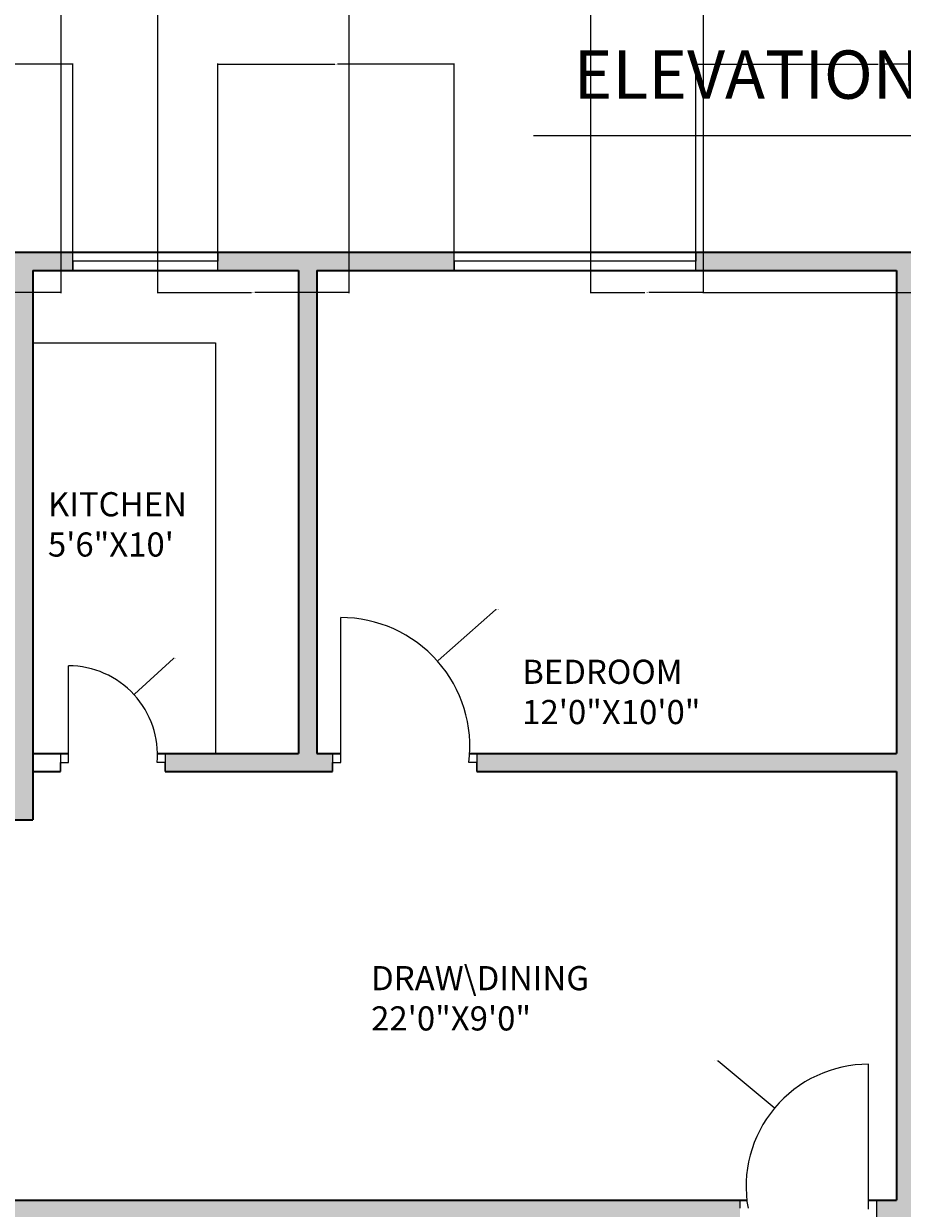
# Model space of a CAD drawing. Units: inches. Extents: x 2314 to 3223, y 1382 to 2735.
# Tile 9 of 14: x 2549 to 2767, y 2144 to 2439. Entities that reach past the tile are written whole.
import ezdxf

# ---------------------------------------------------------------- set-up
doc = ezdxf.new("R2010")
doc.units = ezdxf.units.IN
for name, color, linetype, lineweight in [('A-ANNO-DIMS', 2, 'Continuous', 18), ('A-ANNO-TEXT', 7, 'Continuous', 25), ('A-AREA-IDEN', 7, 'Continuous', 18), ('A-DOOR', 3, 'Continuous', 18), ('A-FLOR-FIXT', 8, 'Continuous', 18), ('A-GLAZ', 4, 'Continuous', 18), ('A-WALL', 7, 'Continuous', 35)]:
    doc.layers.add(name, color=color, linetype=linetype, lineweight=lineweight)
doc.layers.add('A-WALL-PATT', color=251, linetype='Continuous', lineweight=13, true_color=0x636466)
doc.styles.get("Standard").update_dxf_attribs({"font": 'arial.ttf'})
doc.dimstyles.get("Standard").update_dxf_attribs({"dimtxt": 0.18, "dimasz": 0.18, "dimexe": 0.18, "dimexo": 0.0625, "dimgap": 0.09, "dimtad": 0, "dimtih": 1, "dimtoh": 1, "dimdec": 4, "dimzin": 0, "dimdsep": 46, "dimtxsty": 'Standard', "dimcen": 0.09, "dimadec": 0, "dimazin": 0, "dimtfac": 1, "dimtdec": 4, "dimtofl": 0, "dimtmove": 0, "dimatfit": 3, "dimfxl": 1, "dimtolj": 1, "dimtzin": 0, "dimarcsym": 0})

# ---------------------------------------------------------------- blocks, each defined once
blk = doc.blocks.new('WIN-PLAN-60')
for p, q in [((0, 4.5), (0, 0)), ((60, 2.25), (60, 4.5)), ((60, 4.5), (60, 0)), ((0, 0), (0, 2.25)), ((0, 2.25), (60, 2.25))]:
    blk.add_line(p, q)
blk = doc.blocks.new('WIN-PLAN-36')
for p, q in [((0, 36), (4.5, 36)), ((4.5, 36), (2.25, 36)), ((2.25, 36), (2.25, 0)), ((2.25, 0), (0, 0)), ((0, 0), (4.5, 0))]:
    blk.add_line(p, q)
blk = doc.blocks.new('*D41')
at = {"layer": 'A-ANNO-DIMS', "color": 0, "lineweight": -2, "transparency": 16777216}
for p, q in [((2503.33, 2381.85), (2503.33, 2428.66)), ((2503.51, 2428.48), (2531.95, 2428.48)), ((2561.18, 2428.48), (2532.74, 2428.48)), ((2561.36, 2381.85), (2561.36, 2428.66))]:
    blk.add_line(p, q, dxfattribs=at)
at = {"layer": 'A-ANNO-DIMS', "color": 0, "transparency": 16777216}
for points in [[(2503.51, 2428.51), (2503.51, 2428.45), (2503.33, 2428.48)], [(2561.18, 2428.51), (2561.18, 2428.45), (2561.36, 2428.48)]]:
    blk.add_solid(points, dxfattribs=at)
at = {"layer": 'Defpoints', "color": 0, "transparency": 16777216}
for p in [(2561.36, 2428.48), (2503.33, 2381.78), (2561.36, 2381.78)]:
    blk.add_point(p, dxfattribs=at)
at = {"layer": 'A-ANNO-DIMS', "color": 0, "transparency": 16777216, "insert": (2532.35, 2428.48), "char_height": 0.18, "attachment_point": 5}
blk.add_mtext('\\A1;58.03', dxfattribs=at)
blk = doc.blocks.new('*D42')
at = {"layer": 'A-ANNO-DIMS', "color": 0, "lineweight": -2, "transparency": 16777216}
for p, q in [((2597.36, 2381.85), (2597.36, 2428.66)), ((2597.54, 2428.48), (2626.39, 2428.48)), ((2655.88, 2428.48), (2627.04, 2428.48)), ((2656.06, 2381.85), (2656.06, 2428.66))]:
    blk.add_line(p, q, dxfattribs=at)
at = {"layer": 'A-ANNO-DIMS', "color": 0, "transparency": 16777216}
for points in [[(2597.54, 2428.51), (2597.54, 2428.45), (2597.36, 2428.48)], [(2655.88, 2428.51), (2655.88, 2428.45), (2656.06, 2428.48)]]:
    blk.add_solid(points, dxfattribs=at)
at = {"layer": 'Defpoints', "color": 0, "transparency": 16777216}
for p in [(2656.06, 2428.48), (2597.36, 2381.78), (2656.06, 2381.78)]:
    blk.add_point(p, dxfattribs=at)
at = {"layer": 'A-ANNO-DIMS', "color": 0, "transparency": 16777216, "insert": (2626.71, 2428.48), "char_height": 0.18, "attachment_point": 5}
blk.add_mtext('\\A1;58.7', dxfattribs=at)
blk = doc.blocks.new('*D43')
at = {"layer": 'A-ANNO-DIMS', "color": 0, "lineweight": -2, "transparency": 16777216}
for p, q in [((2716.06, 2381.85), (2716.06, 2428.66)), ((2716.24, 2428.48), (2761.31, 2428.48)), ((2807.16, 2428.48), (2762.1, 2428.48)), ((2807.34, 2381.85), (2807.34, 2428.66))]:
    blk.add_line(p, q, dxfattribs=at)
at = {"layer": 'A-ANNO-DIMS', "color": 0, "transparency": 16777216}
for points in [[(2716.24, 2428.51), (2716.24, 2428.45), (2716.06, 2428.48)], [(2807.16, 2428.51), (2807.16, 2428.45), (2807.34, 2428.48)]]:
    blk.add_solid(points, dxfattribs=at)
at = {"layer": 'Defpoints', "color": 0, "transparency": 16777216}
for p in [(2807.34, 2428.48), (2716.06, 2381.78), (2807.34, 2381.78)]:
    blk.add_point(p, dxfattribs=at)
at = {"layer": 'A-ANNO-DIMS', "color": 0, "transparency": 16777216, "insert": (2761.7, 2428.48), "char_height": 0.18, "attachment_point": 5}
blk.add_mtext('\\A1;91.28', dxfattribs=at)
blk = doc.blocks.new('*D53')
at = {"layer": 'A-ANNO-DIMS', "color": 0, "lineweight": -2, "transparency": 16777216}
for p, q in [((2502.93, 2502.62), (2502.93, 2371.63)), ((2558.38, 2502.62), (2558.38, 2371.63)), ((2503.11, 2371.81), (2530.26, 2371.81)), ((2558.2, 2371.81), (2531.05, 2371.81))]:
    blk.add_line(p, q, dxfattribs=at)
at = {"layer": 'A-ANNO-DIMS', "color": 0, "transparency": 16777216}
for points in [[(2503.11, 2371.84), (2503.11, 2371.78), (2502.93, 2371.81)], [(2558.2, 2371.84), (2558.2, 2371.78), (2558.38, 2371.81)]]:
    blk.add_solid(points, dxfattribs=at)
at = {"layer": 'Defpoints', "color": 0, "transparency": 16777216}
for p in [(2502.93, 2502.68), (2558.38, 2502.68), (2558.38, 2371.81)]:
    blk.add_point(p, dxfattribs=at)
at = {"layer": 'A-ANNO-DIMS', "color": 0, "transparency": 16777216, "insert": (2530.66, 2371.81), "char_height": 0.18, "attachment_point": 5}
blk.add_mtext('\\A1;55.45', dxfattribs=at)
blk = doc.blocks.new('*D54')
at = {"layer": 'A-ANNO-DIMS', "color": 0, "lineweight": -2, "transparency": 16777216}
for p, q in [((2582.38, 2502.62), (2582.38, 2371.63)), ((2629.85, 2502.62), (2629.85, 2371.63)), ((2582.56, 2371.81), (2605.72, 2371.81)), ((2629.67, 2371.81), (2606.51, 2371.81))]:
    blk.add_line(p, q, dxfattribs=at)
at = {"layer": 'A-ANNO-DIMS', "color": 0, "transparency": 16777216}
for points in [[(2582.56, 2371.84), (2582.56, 2371.78), (2582.38, 2371.81)], [(2629.67, 2371.84), (2629.67, 2371.78), (2629.85, 2371.81)]]:
    blk.add_solid(points, dxfattribs=at)
at = {"layer": 'Defpoints', "color": 0, "transparency": 16777216}
for p in [(2582.38, 2502.68), (2629.85, 2502.68), (2629.85, 2371.81)]:
    blk.add_point(p, dxfattribs=at)
at = {"layer": 'A-ANNO-DIMS', "color": 0, "transparency": 16777216, "insert": (2606.11, 2371.81), "char_height": 0.18, "attachment_point": 5}
blk.add_mtext('\\A1;47.47', dxfattribs=at)
blk = doc.blocks.new('*D55')
at = {"layer": 'A-ANNO-DIMS', "color": 0, "lineweight": -2, "transparency": 16777216}
for p, q in [((2689.85, 2502.62), (2689.85, 2371.63)), ((2717.89, 2466.62), (2717.89, 2371.63)), ((2690.03, 2371.81), (2703.4, 2371.81)), ((2717.71, 2371.81), (2704.33, 2371.81))]:
    blk.add_line(p, q, dxfattribs=at)
at = {"layer": 'A-ANNO-DIMS', "color": 0, "transparency": 16777216}
for points in [[(2690.03, 2371.84), (2690.03, 2371.78), (2689.85, 2371.81)], [(2717.71, 2371.84), (2717.71, 2371.78), (2717.89, 2371.81)]]:
    blk.add_solid(points, dxfattribs=at)
at = {"layer": 'Defpoints', "color": 0, "transparency": 16777216}
for p in [(2689.85, 2502.68), (2717.89, 2466.68), (2717.89, 2371.81)]:
    blk.add_point(p, dxfattribs=at)
at = {"layer": 'A-ANNO-DIMS', "color": 0, "transparency": 16777216, "insert": (2703.87, 2371.81), "char_height": 0.18, "attachment_point": 5}
blk.add_mtext('\\A1;28.046', dxfattribs=at)
blk = doc.blocks.new('*D56')
at = {"layer": 'A-ANNO-DIMS', "color": 0, "lineweight": -2, "transparency": 16777216}
for p, q in [((2717.89, 2466.62), (2717.89, 2371.63)), ((2822.89, 2466.62), (2822.89, 2371.63)), ((2718.07, 2371.81), (2770.11, 2371.81)), ((2822.71, 2371.81), (2770.67, 2371.81))]:
    blk.add_line(p, q, dxfattribs=at)
at = {"layer": 'A-ANNO-DIMS', "color": 0, "transparency": 16777216}
for points in [[(2718.07, 2371.84), (2718.07, 2371.78), (2717.89, 2371.81)], [(2822.71, 2371.84), (2822.71, 2371.78), (2822.89, 2371.81)]]:
    blk.add_solid(points, dxfattribs=at)
at = {"layer": 'Defpoints', "color": 0, "transparency": 16777216}
for p in [(2717.89, 2466.68), (2822.89, 2466.68), (2822.89, 2371.81)]:
    blk.add_point(p, dxfattribs=at)
at = {"layer": 'A-ANNO-DIMS', "color": 0, "transparency": 16777216, "insert": (2770.39, 2371.81), "char_height": 0.18, "attachment_point": 5}
blk.add_mtext('\\A1;105', dxfattribs=at)
blk = doc.blocks.new('*D66')
at = {"layer": 'A-ANNO-DIMS', "color": 0, "lineweight": -2, "transparency": 16777216}
for p, q in [((2666.3, 2292.96), (2652.02, 2280.33)), ((2666.48, 2292.96), (2666.3, 2292.96)), ((2627.76, 2258.95), (2627.94, 2258.95)), ((2627.85, 2258.86), (2627.85, 2259.04))]:
    blk.add_line(p, q, dxfattribs=at)
at = {"layer": 'A-ANNO-DIMS', "color": 0, "transparency": 16777216}
blk.add_solid([(2652, 2280.35), (2652.04, 2280.3), (2651.88, 2280.21)], dxfattribs=at)
at = {"layer": 'Defpoints', "color": 0, "transparency": 16777216}
for p in [(2651.88, 2280.21), (2627.85, 2258.95)]:
    blk.add_point(p, dxfattribs=at)
at = {"layer": 'A-ANNO-DIMS', "color": 0, "transparency": 16777216, "insert": (2666.96, 2292.96), "char_height": 0.18, "attachment_point": 5}
blk.add_mtext('\\A1;R32.08', dxfattribs=at)
blk = doc.blocks.new('*D68')
at = {"layer": 'A-ANNO-DIMS', "color": 0, "lineweight": -2, "transparency": 16777216}
for p, q in [((2721.4, 2180.88), (2721.58, 2180.88)), ((2721.58, 2180.88), (2735.45, 2169.29)), ((2758.84, 2149.66), (2759.02, 2149.66)), ((2758.93, 2149.57), (2758.93, 2149.75))]:
    blk.add_line(p, q, dxfattribs=at)
at = {"layer": 'A-ANNO-DIMS', "color": 0, "transparency": 16777216}
blk.add_solid([(2735.47, 2169.31), (2735.43, 2169.27), (2735.59, 2169.17)], dxfattribs=at)
at = {"layer": 'Defpoints', "color": 0, "transparency": 16777216}
for p in [(2735.59, 2169.17), (2758.93, 2149.66)]:
    blk.add_point(p, dxfattribs=at)
at = {"layer": 'A-ANNO-DIMS', "color": 0, "transparency": 16777216, "insert": (2720.92, 2180.88), "char_height": 0.18, "attachment_point": 5}
blk.add_mtext('\\A1;R30.42', dxfattribs=at)
blk = doc.blocks.new('*D85')
at = {"layer": 'A-ANNO-DIMS', "color": 0, "lineweight": -2, "transparency": 16777216}
for p, q in [((2586.3, 2280.82), (2576.67, 2271.99)), ((2586.48, 2280.82), (2586.3, 2280.82)), ((2560.17, 2256.96), (2560.35, 2256.96)), ((2560.26, 2256.87), (2560.26, 2257.05))]:
    blk.add_line(p, q, dxfattribs=at)
at = {"layer": 'A-ANNO-DIMS', "color": 0, "transparency": 16777216}
blk.add_solid([(2576.65, 2272.02), (2576.69, 2271.97), (2576.54, 2271.87)], dxfattribs=at)
at = {"layer": 'Defpoints', "color": 0, "transparency": 16777216}
for p in [(2576.54, 2271.87), (2560.26, 2256.96)]:
    blk.add_point(p, dxfattribs=at)
at = {"layer": 'A-ANNO-DIMS', "color": 0, "transparency": 16777216, "insert": (2587.03, 2280.82), "char_height": 0.18, "attachment_point": 5}
blk.add_mtext('\\A1;R22.075', dxfattribs=at)

msp = doc.modelspace()

# ---------------------------------------------------------------- hatches: boundary and pattern name
at = {"layer": 'A-WALL-PATT'}
h = msp.add_hatch(color=256, dxfattribs=at)
h.dxf.hatch_style = 1
h.paths.add_polyline_path([(2443.3302, 2379.5332), (2443.3302, 2381.7832), (2410.3927, 2381.7832), (2410.3927, 2336.7008), (2414.8927, 2336.7008), (2414.8927, 2377.2832), (2443.3302, 2377.2832)])
h.paths.add_polyline_path([(2561.3645, 2379.5332), (2561.3645, 2381.7832), (2503.3302, 2381.7832), (2503.3302, 2377.2832), (2546.8927, 2377.2832), (2546.8927, 2245.2832), (2541.8787, 2245.2832), (2541.8787, 2240.7832), (2551.3927, 2240.7832), (2551.3927, 2377.2832), (2561.3645, 2377.2832)])
h.paths.add_polyline_path([(2656.0607, 2381.7832), (2597.3645, 2381.7832), (2597.3645, 2377.2832), (2617.3927, 2377.2832), (2617.3927, 2257.2832), (2584.2532, 2257.2832), (2584.2532, 2252.7832), (2625.8528, 2252.7832), (2625.8528, 2255.0332), (2625.8528, 2257.2832), (2621.8927, 2257.2832), (2621.8927, 2377.2832), (2656.0607, 2377.2832), (2656.0607, 2379.5332)])
h.paths.add_polyline_path([(2807.3418, 2381.7832), (2716.0607, 2381.7832), (2716.0607, 2377.2832), (2765.8927, 2377.2832), (2765.8927, 2257.2832), (2661.6935, 2257.2832), (2661.6935, 2252.7832), (2765.8927, 2252.7832), (2765.8927, 2146.2832), (2760.9259, 2146.2832), (2760.9259, 2141.8832), (2775.7119, 2141.8832), (2775.7119, 2146.2832), (2770.3927, 2146.2832), (2770.3927, 2252.7832), (2877.684, 2252.7832), (2877.684, 2255.0332), (2877.684, 2257.2832), (2770.3927, 2257.2832), (2770.3927, 2377.2832), (2807.3418, 2377.2832), (2807.3418, 2379.5332)])
h.paths.add_polyline_path([(2937.2118, 2381.7832), (2867.3418, 2381.7832), (2867.3418, 2377.2832), (2914.3927, 2377.2832), (2914.3927, 2257.2832), (2908.4124, 2257.2832), (2908.4124, 2252.7832), (2960.6432, 2252.7832), (2960.6432, 2255.0332), (2960.6432, 2257.2832), (2918.8927, 2257.2832), (2918.8927, 2377.2832), (2937.2118, 2377.2832)])
h.paths.add_polyline_path([(3022.1601, 2381.7832), (2973.2118, 2381.7832), (2973.2118, 2379.5332), (2973.2118, 2377.2832), (2984.8927, 2377.2832), (2984.8927, 2257.2832), (2980.0601, 2257.2832), (2980.0601, 2252.7832), (2984.8927, 2252.7832), (2984.8927, 2240.7832), (2995.668, 2240.7832), (2995.668, 2243.0332), (2995.668, 2245.2832), (2989.3927, 2245.2832), (2989.3927, 2377.2832), (3022.1601, 2377.2832), (3022.1601, 2379.5332)])
h.paths.add_polyline_path([(3125.8927, 2381.7832), (3082.1601, 2381.7832), (3082.1601, 2377.2832), (3121.3927, 2377.2832), (3121.3927, 2334.7388), (3125.8927, 2334.7388)])
h.paths.add_polyline_path([(3125.8927, 2274.7388), (3121.3927, 2274.7388), (3121.3927, 2245.2832), (3066.4832, 2245.2832), (3066.4832, 2240.7832), (3121.3927, 2240.7832), (3121.3927, 2232.1868), (3125.8927, 2232.1868)])
h.paths.add_polyline_path([(3125.8927, 2208.1868), (3121.3927, 2208.1868), (3121.3927, 2198.7832), (3037.3927, 2198.7832), (3037.3927, 2240.7832), (3041.2694, 2240.7832), (3041.2694, 2243.0332), (3041.2694, 2245.2832), (3026.8205, 2245.2832), (3026.8205, 2240.7832), (3032.8927, 2240.7832), (3032.8927, 2190.4022), (3037.3927, 2190.4022), (3037.3927, 2194.2832), (3121.3927, 2194.2832), (3121.3927, 2182.1835), (3125.8927, 2182.1835)])
h.paths.add_polyline_path([(3125.8927, 2158.1835), (3121.3927, 2158.1835), (3121.3927, 2146.2832), (3037.3927, 2146.2832), (3037.3927, 2169.3726), (3035.1427, 2169.3726), (3032.8927, 2169.3726), (3032.8927, 2146.2832), (2812.7301, 2146.2832), (2812.7301, 2144.0832), (2812.7301, 2141.8832), (2818.3927, 2141.8832), (2818.3927, 1970.1316), (2822.8927, 1970.1316), (2822.8927, 1978.8832), (2903.9846, 1978.8832), (2903.9846, 1981.1332), (2903.9846, 1983.3832), (2822.8927, 1983.3832), (2822.8927, 2115.3832), (2851.7162, 2115.3832), (2851.7162, 2117.6332), (2851.7162, 2119.8832), (2822.8927, 2119.8832), (2822.8927, 2141.8832), (3125.8927, 2141.8832)])
h.paths.add_polyline_path([(3125.8927, 2119.8832), (3081.193, 2119.8832), (3081.193, 2115.3832), (3121.3927, 2115.3832), (3121.3927, 2071.8188), (3125.8927, 2071.8188)], flags=17)
h.paths.add_polyline_path([(2989.3927, 2115.3832), (3021.193, 2115.3832), (3021.193, 2117.6332), (3021.193, 2119.8832), (2979.123, 2119.8832), (2979.123, 2115.3832), (2984.8927, 2115.3832), (2984.8927, 2019.3832), (2981.9225, 2019.3832), (2981.9225, 2014.8832), (2984.8927, 2014.8832), (2984.8927, 1983.3832), (2984.8927, 1978.8832), (2989.3927, 1978.8832), (2989.3927, 1983.3832)], flags=17)
h.paths.add_polyline_path([(2947.3927, 2115.3832), (2955.123, 2115.3832), (2955.123, 2117.6332), (2955.123, 2119.8832), (2911.7162, 2119.8832), (2911.7162, 2115.3832), (2942.8927, 2115.3832), (2942.8927, 1983.3832), (2936.7017, 1983.3832), (2936.7017, 1978.8832), (2947.3927, 1978.8832), (2947.3927, 1983.3832), (2947.3927, 2014.8832), (2960.7167, 2014.8832), (2960.7167, 2017.1332), (2960.7167, 2019.3832), (2947.3927, 2019.3832)], flags=17)
h.paths.add_polyline_path([(3037.3927, 1978.8832), (3041.8276, 1978.8832), (3041.8276, 1981.1332), (3041.8276, 1983.3832), (3025.477, 1983.3832), (3025.477, 1978.8832), (3032.8927, 1978.8832), (3032.8927, 1927.1259), (3035.1427, 1927.1259), (3037.3927, 1927.1259)])
h.paths.add_polyline_path([(3125.8927, 2011.8188), (3123.6427, 2011.8188), (3121.3927, 2011.8188), (3121.3927, 1983.3832), (3065, 1983.3832), (3065, 1978.8832), (3121.3927, 1978.8832), (3121.3927, 1970.5932), (3125.8927, 1970.5932)], flags=17)
h.paths.add_polyline_path([(2994.2341, 1983.3832), (2989.3927, 1983.3832), (2989.3927, 1978.8832), (2994.2341, 1978.8832), (2994.2341, 1981.1332)], flags=16)
h.paths.add_polyline_path([(3125.8927, 1946.5932), (3121.3927, 1946.5932), (3121.3927, 1936.8832), (3037.3927, 1936.8832), (3037.3927, 1932.3832), (3121.3927, 1932.3832), (3121.3927, 1919.825), (3125.8927, 1919.825)])
h.paths.add_polyline_path([(3125.8927, 1883.825), (3121.3927, 1883.825), (3121.3927, 1866.3832), (3037.3927, 1866.3832), (3037.3927, 1899.0954), (3035.1427, 1899.0954), (3032.8927, 1899.0954), (3032.8927, 1866.3832), (2822.8927, 1866.3832), (2822.8927, 1938.7212), (2820.6427, 1938.7212), (2818.3927, 1938.7212), (2818.3927, 1786.9239), (2822.8927, 1786.9239), (2822.8927, 1861.8832), (3032.8927, 1861.8832), (3032.8927, 1825.1023), (3037.3927, 1825.1023), (3037.3927, 1861.8832), (3121.3927, 1861.8832), (3121.3927, 1844.6765), (3125.8927, 1844.6765)])
h.paths.add_polyline_path([(3125.8927, 1808.6765), (3121.3927, 1808.6765), (3121.3927, 1795.8832), (3037.3927, 1795.8832), (3037.3927, 1799.4755), (3032.8927, 1799.4755), (3032.8927, 1749.3832), (3026.5034, 1749.3832), (3026.5034, 1744.8832), (3032.8927, 1744.8832), (3034.9255, 1744.8832), (3043.1326, 1744.8832), (3043.1326, 1747.1332), (3043.1326, 1749.3832), (3037.3927, 1749.3832), (3037.3927, 1791.3832), (3121.3927, 1791.3832), (3121.3927, 1783.3103), (3125.8927, 1783.3103)])
h.paths.add_polyline_path([(3125.8927, 1759.3103), (3121.3927, 1759.3103), (3121.3927, 1749.3832), (3065.1845, 1749.3832), (3065.1845, 1744.8832), (3121.3927, 1744.8832), (3121.3927, 1709.3573), (3125.8927, 1709.3573)])
h.paths.add_polyline_path([(3125.8927, 1649.3573), (3121.3927, 1649.3573), (3121.3927, 1612.8832), (3095.116, 1612.8832), (3095.116, 1608.3832), (3125.8927, 1608.3832)])
h.paths.add_polyline_path([(3035.116, 1612.8832), (2993.8927, 1612.8832), (2993.8927, 1744.8832), (2998.7409, 1744.8832), (2998.7409, 1749.3832), (2989.3927, 1749.3832), (2989.3927, 1744.8832), (2989.3927, 1701.3832), (2972.8226, 1701.3832), (2972.8226, 1696.8832), (2989.3927, 1696.8832), (2989.3927, 1612.8832), (2978.2225, 1612.8832), (2978.2225, 1608.3832), (3035.116, 1608.3832), (3035.116, 1610.6332)])
h.paths.add_polyline_path([(2947.3927, 1696.8832), (2950.7566, 1696.8832), (2950.7566, 1699.1332), (2950.7566, 1701.3832), (2947.3927, 1701.3832), (2947.3927, 1744.8832), (2947.3927, 1749.3832), (2937.649, 1749.3832), (2937.649, 1744.8832), (2942.8927, 1744.8832), (2942.8927, 1612.8832), (2907.783, 1612.8832), (2907.783, 1608.3832), (2954.2225, 1608.3832), (2954.2225, 1610.6332), (2954.2225, 1612.8832), (2947.3927, 1612.8832)])
h.paths.add_polyline_path([(2822.8927, 1744.8832), (2905.3491, 1744.8832), (2905.3491, 1747.1332), (2905.3491, 1749.3832), (2822.8927, 1749.3832), (2822.8927, 1756.9185), (2818.3927, 1756.9185), (2818.3927, 1612.8832), (2818.3927, 1569.1205), (2722.3927, 1569.1205), (2722.3927, 1612.8832), (2722.3927, 1756.9185), (2717.8927, 1756.9185), (2717.8927, 1750.0143), (2633.6297, 1750.0143), (2633.6437, 1745.2665), (2717.8927, 1745.5143), (2717.8927, 1612.8832), (2689.8467, 1612.8832), (2689.8467, 1608.3832), (2717.8927, 1608.3832), (2717.8927, 1564.6205), (2722.3927, 1564.6205), (2822.8927, 1564.6205), (2822.8927, 1569.1205), (2822.8927, 1608.3832), (2847.783, 1608.3832), (2847.783, 1610.6332), (2847.783, 1612.8832), (2822.8927, 1612.8832)])
h.paths.add_polyline_path([(2629.8467, 1612.8832), (2597.8927, 1612.8832), (2597.8927, 1744.8832), (2597.8927, 1745.1613), (2601.5887, 1745.1721), (2601.5816, 1747.5932), (2601.5745, 1750.0143), (2593.3927, 1750.0143), (2593.3927, 1744.8832), (2593.3927, 1713.3832), (2589.7588, 1713.3832), (2589.7588, 1708.8832), (2593.3927, 1708.8832), (2593.3927, 1612.8832), (2582.3793, 1612.8832), (2582.3793, 1608.3832), (2629.8467, 1608.3832), (2629.8467, 1610.6332)])
h.paths.add_polyline_path([(2551.3927, 1708.8832), (2567.6776, 1708.8832), (2567.6776, 1711.1332), (2567.6776, 1713.3832), (2551.3927, 1713.3832), (2551.3927, 1744.8832), (2551.3927, 1750.0143), (2543.5657, 1750.0143), (2543.5657, 1747.5079), (2543.5657, 1745.0014), (2546.8927, 1745.0112), (2546.8927, 1744.8832), (2546.8927, 1612.8832), (2502.9339, 1612.8832), (2502.9339, 1608.3832), (2558.3793, 1608.3832), (2558.3793, 1610.6332), (2558.3793, 1612.8832), (2551.3927, 1612.8832)])
h.paths.add_polyline_path([(2414.8927, 1656.2547), (2410.3927, 1656.2547), (2410.3927, 1608.3832), (2442.9339, 1608.3832), (2442.9339, 1610.6332), (2442.9339, 1612.8832), (2414.8927, 1612.8832)])
h.paths.add_polyline_path([(2414.8927, 1744.8832), (2468.8906, 1744.8832), (2468.8906, 1747.1332), (2468.8906, 1749.3832), (2414.8927, 1749.3832), (2414.8927, 1757.7622), (2410.3927, 1757.7622), (2410.3927, 1716.2547), (2414.8927, 1716.2547)])
h.paths.add_polyline_path([(2414.8927, 1791.3832), (2498.8927, 1791.3832), (2498.8927, 1749.3832), (2492.9799, 1749.3832), (2492.9799, 1744.8832), (2498.8927, 1744.8832), (2503.3927, 1744.8832), (2508.0135, 1744.8968), (2508.0059, 1747.4556), (2507.9984, 1750.0143), (2503.3927, 1750.0143), (2503.3927, 1802.6362), (2501.1427, 1802.6362), (2498.8927, 1802.6362), (2498.8927, 1795.8832), (2414.8927, 1795.8832), (2414.8927, 1808.0943), (2410.3927, 1808.0943), (2410.3927, 1781.7622), (2414.8927, 1781.7622)])
h.paths.add_polyline_path([(2722.3927, 1937.589), (2720.1427, 1937.589), (2717.8927, 1937.589), (2717.8927, 1866.3832), (2503.3927, 1866.3832), (2503.3927, 1896.3484), (2498.8927, 1896.3484), (2498.8927, 1866.3832), (2414.8927, 1866.3832), (2414.8927, 1882.1496), (2410.3927, 1882.1496), (2410.3927, 1844.0943), (2414.8927, 1844.0943), (2414.8927, 1861.8832), (2498.8927, 1861.8832), (2498.8927, 1831.4783), (2501.1427, 1831.4783), (2503.3927, 1831.4783), (2503.3927, 1861.8832), (2717.8927, 1861.8832), (2717.8927, 1786.9239), (2722.3927, 1786.9239)])
h.paths.add_polyline_path([(2414.8927, 1932.3832), (2498.8927, 1932.3832), (2498.8927, 1924.7883), (2503.3927, 1924.7883), (2503.3927, 1978.8832), (2505.8599, 1978.8832), (2505.8599, 1981.1332), (2505.8599, 1983.3832), (2493.3697, 1983.3832), (2493.3697, 1978.8832), (2498.8927, 1978.8832), (2498.8927, 1936.8832), (2414.8927, 1936.8832), (2414.8927, 1943.2834), (2410.3927, 1943.2834), (2410.3927, 1918.1496), (2414.8927, 1918.1496)])
h.paths.add_polyline_path([(2414.8927, 2020.3133), (2412.6427, 2020.3133), (2410.3927, 2020.3133), (2410.3927, 1967.2834), (2414.8927, 1967.2834), (2414.8927, 1978.8832), (2468.8513, 1978.8832), (2468.8513, 1981.1332), (2468.8513, 1983.3832), (2414.8927, 1983.3832)])
h.paths.add_polyline_path([(2414.8927, 2115.3832), (2453.004, 2115.3832), (2453.004, 2117.6332), (2453.004, 2119.8832), (2410.3927, 2119.8832), (2410.3927, 2080.3133), (2414.8927, 2080.3133)], flags=17)
h.paths.add_polyline_path([(2559.0969, 2117.6332), (2559.0969, 2119.8832), (2513.004, 2119.8832), (2513.004, 2115.3832), (2546.8927, 2115.3832), (2546.8927, 1983.3832), (2542.7531, 1983.3832), (2542.7531, 1978.8832), (2551.3927, 1978.8832), (2551.3927, 2014.8832), (2570.3098, 2014.8832), (2570.3098, 2017.1332), (2570.3098, 2019.3832), (2551.3927, 2019.3832), (2551.3927, 2115.3832), (2559.0969, 2115.3832)], flags=17)
h.paths.add_polyline_path([(2628.5073, 2117.6332), (2628.5073, 2119.8832), (2583.0969, 2119.8832), (2583.0969, 2115.3832), (2593.3927, 2115.3832), (2593.3927, 2019.3832), (2590.2108, 2019.3832), (2590.2108, 2014.8832), (2593.3927, 2014.8832), (2593.3927, 1978.8832), (2601.5907, 1978.8832), (2601.5907, 1981.1332), (2601.5907, 1983.3832), (2597.8927, 1983.3832), (2597.8927, 2115.3832), (2628.5073, 2115.3832)], flags=17)
h.paths.add_polyline_path([(2722.3927, 2141.8832), (2726.9871, 2141.8832), (2726.9871, 2144.2705), (2726.9871, 2146.2832), (2503.3927, 2146.2832), (2503.3927, 2168.2161), (2501.1427, 2168.2161), (2498.8927, 2168.2161), (2498.8927, 2146.2832), (2414.8927, 2146.2832), (2414.8927, 2156.5041), (2410.3927, 2156.5041), (2410.3927, 2141.8832), (2717.8927, 2141.8832), (2717.8927, 2119.8832), (2688.5073, 2119.8832), (2688.5073, 2115.3832), (2717.8927, 2115.3832), (2717.8927, 1983.3832), (2633.2454, 1983.3832), (2633.2454, 1978.8832), (2717.8927, 1978.8832), (2717.8927, 1970.1316), (2720.1427, 1970.1316), (2722.3927, 1970.1316)])
h.paths.add_polyline_path([(2557.3704, 1462.9278), (2940.0934, 1462.9278), (2940.0934, 1512.3848), (2557.3704, 1512.3848)], flags=9)
h.paths.add_polyline_path([(2846.2527, 1703.1384), (2892.8612, 1703.1384), (2892.8612, 1725.5272), (2846.2527, 1725.5272)], flags=25)
h.paths.add_polyline_path([(2885.6102, 1812.1147), (2946.1505, 1812.1147), (2946.1505, 1834.5035), (2885.6102, 1834.5035)], flags=25)
h.paths.add_polyline_path([(2885.6102, 1884.183), (2946.1505, 1884.183), (2946.1505, 1906.5718), (2885.6102, 1906.5718)], flags=25)
h.paths.add_polyline_path([(3066.365, 1705.5431), (3112.9735, 1705.5431), (3112.9735, 1727.9319), (3066.365, 1727.9319)], flags=9)
h.paths.add_polyline_path([(3061.8255, 1887.7513), (3101.6154, 1887.7513), (3101.6154, 1910.1401), (3061.8255, 1910.1401)], flags=25)
h.paths.add_polyline_path([(3063.3679, 1816.2121), (3103.1578, 1816.2121), (3103.1578, 1838.6009), (3063.3679, 1838.6009)], flags=25)
h.paths.add_polyline_path([(3053.3743, 1768.416), (3107.1329, 1768.416), (3107.1329, 1790.8048), (3053.3743, 1790.8048)], flags=25)
h.paths.add_polyline_path([(3061.6068, 1943.822), (3115.3653, 1943.822), (3115.3653, 1966.2109), (3061.6068, 1966.2109)], flags=9)
h.paths.add_polyline_path([(2745.0978, 1763.6604), (2797.9354, 1763.6604), (2797.9354, 1776.0247), (2745.0978, 1776.0247)], flags=9)
h.paths.add_polyline_path([(2574.2135, 1819.2586), (2634.7538, 1819.2586), (2634.7538, 1841.6474), (2574.2135, 1841.6474)], flags=25)
h.paths.add_polyline_path([(2574.2135, 1891.3269), (2634.7538, 1891.3269), (2634.7538, 1913.7157), (2574.2135, 1913.7157)], flags=25)
h.paths.add_polyline_path([(2638.4466, 1702.43), (2685.0551, 1702.43), (2685.0551, 1724.8188), (2638.4466, 1724.8188)], flags=25)
h.paths.add_polyline_path([(2435.9715, 1697.1215), (2482.5799, 1697.1215), (2482.5799, 1719.5103), (2435.9715, 1719.5103)], flags=9)
h.paths.add_polyline_path([(2431.2046, 1893.7833), (2470.9945, 1893.7833), (2470.9945, 1916.1721), (2431.2046, 1916.1721)], flags=25)
h.paths.add_polyline_path([(2439.8144, 1817.2116), (2479.6043, 1817.2116), (2479.6043, 1839.6004), (2439.8144, 1839.6004)], flags=25)
h.paths.add_polyline_path([(2441.2607, 1753.0942), (2495.0192, 1753.0942), (2495.0192, 1775.483), (2441.2607, 1775.483)], flags=25)
h.paths.add_polyline_path([(2421.216, 1945.3109), (2474.9746, 1945.3109), (2474.9746, 1967.6997), (2421.216, 1967.6997)], flags=25)
h.paths.add_polyline_path([(2585.4464, 1627.5703), (2585.4464, 1679), (2563.0576, 1679), (2563.0576, 1627.5703)], flags=9)
h.paths.add_polyline_path([(2978.3497, 1618.7039), (2978.3497, 1670.1337), (2955.9609, 1670.1337), (2955.9609, 1618.7039)], flags=9)
h.paths.add_polyline_path([(2975.9502, 2041.7828), (2975.9502, 2093.2125), (2953.5614, 2093.2125), (2953.5614, 2041.7828)], flags=25)
h.paths.add_polyline_path([(2835.6537, 1989.2068), (2882.2621, 1989.2068), (2882.2621, 2011.5956), (2835.6537, 2011.5956)], flags=25)
h.paths.add_polyline_path([(2649.3769, 1997.5659), (2695.9853, 1997.5659), (2695.9853, 2019.9547), (2649.3769, 2019.9547)], flags=25)
h.paths.add_polyline_path([(2579.9087, 2040.3429), (2579.9087, 2091.7726), (2557.5198, 2091.7726), (2557.5198, 2040.3429)], flags=25)
h.paths.add_polyline_path([(2783.2404, 1883.1956), (2783.2404, 2067.1369), (2764.694, 2067.1369), (2764.694, 1883.1956)], flags=9)
h.paths.add_polyline_path([(3055.8435, 1993.5571), (3102.4519, 1993.5571), (3102.4519, 2015.9459), (3055.8435, 2015.9459)], flags=25)
h.paths.add_polyline_path([(2423.6009, 1984.6082), (2470.2094, 1984.6082), (2470.2094, 2006.997), (2423.6009, 2006.997)], flags=25)
h.paths.add_polyline_path([(2973.4115, 2123.1668), (3013.1319, 2123.1668), (3013.1319, 2135.531), (2973.4115, 2135.531)], flags=25)
h.paths.add_polyline_path([(2534.3846, 2124.6231), (2574.105, 2124.6231), (2574.105, 2136.9874), (2534.3846, 2136.9874)], flags=25)
h.paths.add_polyline_path([(2829.1368, 2188.1931), (2889.411, 2188.1931), (2889.411, 2210.5819), (2829.1368, 2210.5819)], flags=9)
h.paths.add_polyline_path([(2633.2547, 2185.0437), (2693.5289, 2185.0437), (2693.5289, 2207.4325), (2633.2547, 2207.4325)], flags=9)
h.paths.add_polyline_path([(2445.1812, 2167.0395), (2496.611, 2167.0395), (2496.611, 2189.4284), (2445.1812, 2189.4284)], flags=9)
h.paths.add_polyline_path([(2429.1678, 2194.5482), (2480.5975, 2194.5482), (2480.5975, 2216.937), (2429.1678, 2216.937)], flags=9)
h.paths.add_polyline_path([(3060.1138, 2158.1056), (3111.5436, 2158.1056), (3111.5436, 2180.4944), (3060.1138, 2180.4944)], flags=9)
h.paths.add_polyline_path([(3055.6824, 2201.2631), (3107.1122, 2201.2631), (3107.1122, 2223.652), (3055.6824, 2223.652)], flags=25)
h.paths.add_polyline_path([(3044.3482, 2257.7345), (3090.9567, 2257.7345), (3090.9567, 2280.1233), (3044.3482, 2280.1233)], flags=9)
h.paths.add_polyline_path([(2942.5437, 2306.9625), (2982.3336, 2306.9625), (2982.3336, 2329.3513), (2942.5437, 2329.3513)], flags=9)
h.paths.add_polyline_path([(2799.5865, 2259.1663), (2846.195, 2259.1663), (2846.195, 2281.5551), (2799.5865, 2281.5551)], flags=25)
h.paths.add_polyline_path([(2670.4998, 2261.1493), (2717.1082, 2261.1493), (2717.1082, 2283.5381), (2670.4998, 2283.5381)], flags=25)
h.paths.add_polyline_path([(2553.0333, 2302.7735), (2592.8232, 2302.7735), (2592.8232, 2325.1624), (2553.0333, 2325.1624)], flags=9)
h.paths.add_polyline_path([(2432.0288, 2268.6489), (2478.6372, 2268.6489), (2478.6372, 2291.0377), (2432.0288, 2291.0377)], flags=9)
h = msp.add_hatch(color=256, dxfattribs=at)
h.dxf.hatch_style = 1
h.paths.add_polyline_path([(2503.3927, 2240.7832), (2507.7952, 2240.7832), (2507.7952, 2245.2832), (2496.4262, 2245.2832), (2496.4262, 2243.0332), (2496.4262, 2240.7832), (2498.8927, 2240.7832), (2498.8927, 2198.7832), (2414.8927, 2198.7832), (2414.8927, 2206.5718), (2410.3927, 2206.5718), (2410.3927, 2180.5041), (2412.6427, 2180.5041), (2414.8927, 2180.5041), (2414.8927, 2194.2832), (2498.8927, 2194.2832), (2498.8927, 2191.0069), (2503.3927, 2191.0069)])
h.paths.add_polyline_path([(2414.8927, 2276.7008), (2410.3927, 2276.7008), (2410.3927, 2230.5718), (2414.8927, 2230.5718), (2414.8927, 2240.7832), (2474.2564, 2240.7832), (2474.2564, 2243.0332), (2474.2564, 2245.2832), (2414.8927, 2245.2832)])
h.paths.add_polyline_path([(2557.3704, 1462.9278), (2940.0934, 1462.9278), (2940.0934, 1512.3848), (2557.3704, 1512.3848)], flags=9)
h.paths.add_polyline_path([(2846.2527, 1703.1384), (2892.8612, 1703.1384), (2892.8612, 1725.5272), (2846.2527, 1725.5272)], flags=9)
h.paths.add_polyline_path([(2885.6102, 1812.1147), (2946.1505, 1812.1147), (2946.1505, 1834.5035), (2885.6102, 1834.5035)], flags=9)
h.paths.add_polyline_path([(2885.6102, 1884.183), (2946.1505, 1884.183), (2946.1505, 1906.5718), (2885.6102, 1906.5718)], flags=9)
h.paths.add_polyline_path([(3066.365, 1705.5431), (3112.9735, 1705.5431), (3112.9735, 1727.9319), (3066.365, 1727.9319)], flags=9)
h.paths.add_polyline_path([(3061.8255, 1887.7513), (3101.6154, 1887.7513), (3101.6154, 1910.1401), (3061.8255, 1910.1401)], flags=9)
h.paths.add_polyline_path([(3063.3679, 1816.2121), (3103.1578, 1816.2121), (3103.1578, 1838.6009), (3063.3679, 1838.6009)], flags=9)
h.paths.add_polyline_path([(3053.3743, 1768.416), (3107.1329, 1768.416), (3107.1329, 1790.8048), (3053.3743, 1790.8048)], flags=9)
h.paths.add_polyline_path([(3061.6068, 1943.822), (3115.3653, 1943.822), (3115.3653, 1966.2109), (3061.6068, 1966.2109)], flags=9)
h.paths.add_polyline_path([(2745.0978, 1763.6604), (2797.9354, 1763.6604), (2797.9354, 1776.0247), (2745.0978, 1776.0247)], flags=9)
h.paths.add_polyline_path([(2574.2135, 1819.2586), (2634.7538, 1819.2586), (2634.7538, 1841.6474), (2574.2135, 1841.6474)], flags=9)
h.paths.add_polyline_path([(2574.2135, 1891.3269), (2634.7538, 1891.3269), (2634.7538, 1913.7157), (2574.2135, 1913.7157)], flags=9)
h.paths.add_polyline_path([(2638.4466, 1702.43), (2685.0551, 1702.43), (2685.0551, 1724.8188), (2638.4466, 1724.8188)], flags=9)
h.paths.add_polyline_path([(2435.9715, 1697.1215), (2482.5799, 1697.1215), (2482.5799, 1719.5103), (2435.9715, 1719.5103)], flags=9)
h.paths.add_polyline_path([(2431.2046, 1893.7833), (2470.9945, 1893.7833), (2470.9945, 1916.1721), (2431.2046, 1916.1721)], flags=9)
h.paths.add_polyline_path([(2439.8144, 1817.2116), (2479.6043, 1817.2116), (2479.6043, 1839.6004), (2439.8144, 1839.6004)], flags=9)
h.paths.add_polyline_path([(2441.2607, 1753.0942), (2495.0192, 1753.0942), (2495.0192, 1775.483), (2441.2607, 1775.483)], flags=9)
h.paths.add_polyline_path([(2421.216, 1945.3109), (2474.9746, 1945.3109), (2474.9746, 1967.6997), (2421.216, 1967.6997)], flags=9)
h.paths.add_polyline_path([(2585.4464, 1627.5703), (2585.4464, 1679), (2563.0576, 1679), (2563.0576, 1627.5703)], flags=9)
h.paths.add_polyline_path([(2978.3497, 1618.7039), (2978.3497, 1670.1337), (2955.9609, 1670.1337), (2955.9609, 1618.7039)], flags=9)
h.paths.add_polyline_path([(2975.9502, 2041.7828), (2975.9502, 2093.2125), (2953.5614, 2093.2125), (2953.5614, 2041.7828)], flags=9)
h.paths.add_polyline_path([(2835.6537, 1989.2068), (2882.2621, 1989.2068), (2882.2621, 2011.5956), (2835.6537, 2011.5956)], flags=9)
h.paths.add_polyline_path([(2649.3769, 1997.5659), (2695.9853, 1997.5659), (2695.9853, 2019.9547), (2649.3769, 2019.9547)], flags=9)
h.paths.add_polyline_path([(2579.9087, 2040.3429), (2579.9087, 2091.7726), (2557.5198, 2091.7726), (2557.5198, 2040.3429)], flags=9)
h.paths.add_polyline_path([(2783.2404, 1883.1956), (2783.2404, 2067.1369), (2764.694, 2067.1369), (2764.694, 1883.1956)], flags=9)
h.paths.add_polyline_path([(3055.8435, 1993.5571), (3102.4519, 1993.5571), (3102.4519, 2015.9459), (3055.8435, 2015.9459)], flags=9)
h.paths.add_polyline_path([(2423.6009, 1984.6082), (2470.2094, 1984.6082), (2470.2094, 2006.997), (2423.6009, 2006.997)], flags=9)
h.paths.add_polyline_path([(2973.4115, 2123.1668), (3013.1319, 2123.1668), (3013.1319, 2135.531), (2973.4115, 2135.531)], flags=9)
h.paths.add_polyline_path([(2534.3846, 2124.6231), (2574.105, 2124.6231), (2574.105, 2136.9874), (2534.3846, 2136.9874)], flags=9)
h.paths.add_polyline_path([(2829.1368, 2188.1931), (2889.411, 2188.1931), (2889.411, 2210.5819), (2829.1368, 2210.5819)], flags=9)
h.paths.add_polyline_path([(2633.2547, 2185.0437), (2693.5289, 2185.0437), (2693.5289, 2207.4325), (2633.2547, 2207.4325)], flags=9)
h.paths.add_polyline_path([(2445.1812, 2167.0395), (2496.611, 2167.0395), (2496.611, 2189.4284), (2445.1812, 2189.4284)], flags=9)
h.paths.add_polyline_path([(2429.1678, 2208.3022), (2480.5975, 2208.3022), (2480.5975, 2230.691), (2429.1678, 2230.691)], flags=25)
h.paths.add_polyline_path([(3060.1138, 2158.1056), (3111.5436, 2158.1056), (3111.5436, 2180.4944), (3060.1138, 2180.4944)], flags=9)
h.paths.add_polyline_path([(3055.6824, 2201.2631), (3107.1122, 2201.2631), (3107.1122, 2223.652), (3055.6824, 2223.652)], flags=9)
h.paths.add_polyline_path([(3044.3482, 2257.7345), (3090.9567, 2257.7345), (3090.9567, 2280.1233), (3044.3482, 2280.1233)], flags=9)
h.paths.add_polyline_path([(2942.5437, 2306.9625), (2982.3336, 2306.9625), (2982.3336, 2329.3513), (2942.5437, 2329.3513)], flags=9)
h.paths.add_polyline_path([(2799.5865, 2259.1663), (2846.195, 2259.1663), (2846.195, 2281.5551), (2799.5865, 2281.5551)], flags=9)
h.paths.add_polyline_path([(2670.4998, 2261.1493), (2717.1082, 2261.1493), (2717.1082, 2283.5381), (2670.4998, 2283.5381)], flags=9)
h.paths.add_polyline_path([(2553.0333, 2302.7735), (2592.8232, 2302.7735), (2592.8232, 2325.1624), (2553.0333, 2325.1624)], flags=9)
h.paths.add_polyline_path([(2432.0288, 2268.6489), (2478.6372, 2268.6489), (2478.6372, 2291.0377), (2432.0288, 2291.0377)], flags=9)

# ---------------------------------------------------------------- linework, layer by layer
at = {"layer": 'A-ANNO-TEXT'}
msp.add_line((2675.75, 2410.8121), (2785.7373, 2410.8121), dxfattribs=at)
at = {"layer": 'A-DOOR'}
for p, q in [((2627.8528, 2255.0332), (2627.8528, 2291.0332)), ((2560.262, 2255.0332), (2560.262, 2279.0332)), ((2558.262, 2257.2832), (2558.262, 2252.7832)), ((2584.2532, 2257.2832), (2584.2532, 2252.7832)), ((2625.8528, 2257.2832), (2625.8528, 2252.7832)), ((2661.6935, 2257.2832), (2661.6935, 2252.7832)), ((2558.262, 2252.7832), (2558.262, 2255.0332)), ((2558.262, 2255.0332), (2560.262, 2255.0332)), ((2584.2532, 2255.0332), (2582.2532, 2255.0332)), ((2584.2532, 2252.7832), (2584.2532, 2255.0332)), ((2625.8528, 2252.7832), (2625.8528, 2255.0332)), ((2625.8528, 2255.0332), (2627.8528, 2255.0332)), ((2661.6935, 2255.0332), (2659.6935, 2255.0332)), ((2661.6935, 2252.7832), (2661.6935, 2255.0332)), ((2758.9259, 2144.0832), (2758.9259, 2180.0832)), ((2726.9871, 2146.2832), (2726.9871, 2144.2705)), ((2760.9259, 2146.2832), (2760.9259, 2141.8832))]:
    msp.add_line(p, q, dxfattribs=at)
for centre, radius, start, end in [((2627.8528, 2258.9523), 32.0809, 352.9831, 90), ((2560.262, 2256.958), 22.0752, 354.997892, 90), ((2758.9259, 2149.6627), 30.4205, 90, 190.209835)]:
    msp.add_arc(centre, radius, start, end, dxfattribs=at)
at = {"layer": 'A-FLOR-FIXT'}
for p, q in [((2551.3927, 2359.2363), (2596.7587, 2359.2363)), ((2596.7587, 2359.2363), (2596.7587, 2257.2832))]:
    msp.add_line(p, q, dxfattribs=at)
at = {"layer": 'A-WALL'}
for p, q in [((2410.3927, 2381.7832), (3125.8927, 2381.7832)), ((2551.3927, 2377.2832), (2551.3927, 2240.7832)), ((2551.3927, 2377.2832), (2617.3927, 2377.2832)), ((2617.3927, 2377.2832), (2617.3927, 2257.2832)), ((2621.8927, 2377.2832), (2621.8927, 2257.2832)), ((2621.8927, 2377.2832), (2765.8927, 2377.2832)), ((2765.8927, 2377.2832), (2765.8927, 2257.2832)), ((2551.3927, 2257.2832), (2560.262, 2257.2832)), ((2582.3349, 2257.2832), (2617.3927, 2257.2832)), ((2621.8927, 2257.2832), (2627.8528, 2257.2832)), ((2659.8903, 2257.2832), (2765.8927, 2257.2832)), ((2551.3927, 2252.7832), (2558.262, 2252.7832)), ((2584.2532, 2252.7832), (2625.8528, 2252.7832)), ((2661.6935, 2252.7832), (2765.8927, 2252.7832)), ((2765.8927, 2252.7832), (2765.8927, 2146.2832)), ((2541.8787, 2240.7832), (2551.3927, 2240.7832)), ((2503.3927, 2146.2832), (2728.6937, 2146.2832)), ((2758.9259, 2146.2832), (2765.8927, 2146.2832))]:
    msp.add_line(p, q, dxfattribs=at)

# ---------------------------------------------------------------- block references
at = {"layer": 'A-GLAZ', "extrusion": (0, 0, -1), "zscale": -1, "rotation": 90}
msp.add_blockref('WIN-PLAN-36', (-2561.3645, 2377.2832), dxfattribs=at)
at = {"layer": 'A-GLAZ', "rotation": 180}
msp.add_blockref('WIN-PLAN-60', (2716.0607, 2381.7832), dxfattribs=at)

# ---------------------------------------------------------------- texts
at = {"layer": 'A-ANNO-TEXT', "insert": (2685.687, 2431.9165), "char_height": 12, "attachment_point": 1}
msp.add_mtext_dynamic_manual_height_columns('ELEVATION', width=331.233746, gutter_width=12.5, heights=[0], dxfattribs=at)
at = {"layer": 'A-AREA-IDEN', "char_height": 6, "attachment_point": 1}
for s, width, insert in [('KITCHEN\\P5\'6"X10\'', 91.281907, (2555.1472, 2322.1767)), ('BEDROOM\\P12\'0"X10\'0"', 89.719354, (2672.9125, 2280.5565)), ('DRAW\\\\DINING\\P22\'0"X9\'0"', 93.899013, (2635.4014, 2204.4469))]:
    msp.add_mtext_dynamic_manual_height_columns(s, width=width, gutter_width=12.5, heights=[0], dxfattribs=dict(at, insert=insert))

# ---------------------------------------------------------------- dimensions: what is measured, and where the dimension line sits
at = {"layer": 'A-ANNO-DIMS'}
for base, p1, p2, override, picture, middle in [((2558.3793, 2371.8121), (2502.9339, 2502.6793), (2558.3793, 2502.6793), {"dimdec": 2, "dimlfac": 1, "dimrnd": 0, "dimzin": 0, "dimdsep": 46, "dimlunit": 2}, '*D53', (2530.6566, 2371.8121)), ((2629.8467, 2371.8121), (2582.3793, 2502.6793), (2629.8467, 2502.6793), {"dimdec": 2, "dimlfac": 1, "dimrnd": 0, "dimzin": 0, "dimdsep": 46, "dimlunit": 2}, '*D54', (2606.113, 2371.8121)), ((2717.8927, 2371.8121), (2689.8467, 2502.6793), (2717.8927, 2466.6793), {"dimdec": 3, "dimlfac": 1, "dimrnd": 0, "dimzin": 0, "dimdsep": 46, "dimlunit": 2}, '*D55', (2703.8697, 2371.8121)), ((2822.8927, 2371.8121), (2717.8927, 2466.6793), (2822.8927, 2466.6793), {"dimdec": 0, "dimlfac": 1, "dimrnd": 0, "dimzin": 0, "dimdsep": 46, "dimlunit": 2}, '*D56', (2770.3927, 2371.8121)), ((2561.3645, 2428.4832), (2503.3302, 2381.7832), (2561.3645, 2381.7832), {"dimdec": 2, "dimlfac": 1, "dimrnd": 0, "dimzin": 0, "dimdsep": 46, "dimlunit": 2}, '*D41', (2532.3474, 2428.4832)), ((2656.0607, 2428.4832), (2597.3645, 2381.7832), (2656.0607, 2381.7832), {"dimdec": 1, "dimlfac": 1, "dimrnd": 0, "dimzin": 0, "dimdsep": 46, "dimlunit": 2}, '*D42', (2626.7126, 2428.4832)), ((2807.3418, 2428.4832), (2716.0607, 2381.7832), (2807.3418, 2381.7832), {"dimdec": 2, "dimlfac": 1, "dimrnd": 0, "dimzin": 0, "dimdsep": 46, "dimlunit": 2}, '*D43', (2761.7012, 2428.4832))]:
    dim = msp.add_linear_dim(base=base, p1=p1, p2=p2, dimstyle='Standard', override=override, dxfattribs=at)
    dim.commit()
    dim.dimension.update_dxf_attribs({"geometry": picture, "text_midpoint": middle})
for center, mpoint, override, picture, middle in [((2627.8528, 2258.9523), (2651.8832, 2280.2062), {"dimdec": 2, "dimlfac": 1, "dimrnd": 0, "dimzin": 0, "dimdsep": 46, "dimlunit": 2}, '*D66', (2666.9615, 2292.9585)), ((2560.262, 2256.958), (2576.5377, 2271.8717), {"dimdec": 3, "dimlfac": 1, "dimrnd": 0, "dimzin": 0, "dimdsep": 46, "dimlunit": 2}, '*D85', (2587.0335, 2280.8199)), ((2758.9259, 2149.6627), (2735.5868, 2169.1741), {"dimdec": 2, "dimlfac": 1, "dimrnd": 0, "dimzin": 0, "dimdsep": 46, "dimlunit": 2}, '*D68', (2720.9245, 2180.881))]:
    dim = msp.add_radius_dim(center=center, mpoint=mpoint, dimstyle='Standard', override=override, dxfattribs=at)
    dim.commit()
    dim.dimension.update_dxf_attribs({"geometry": picture, "text_midpoint": middle, "dimtype": 164})

doc.saveas('drawing.dxf')
